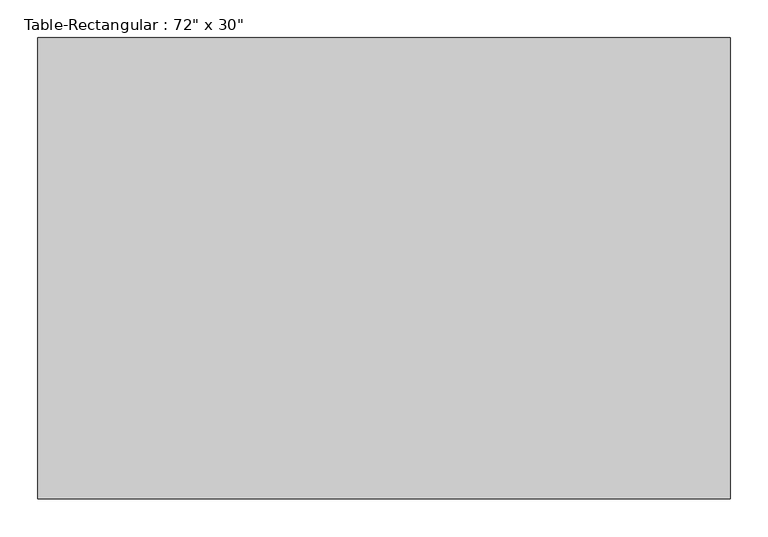
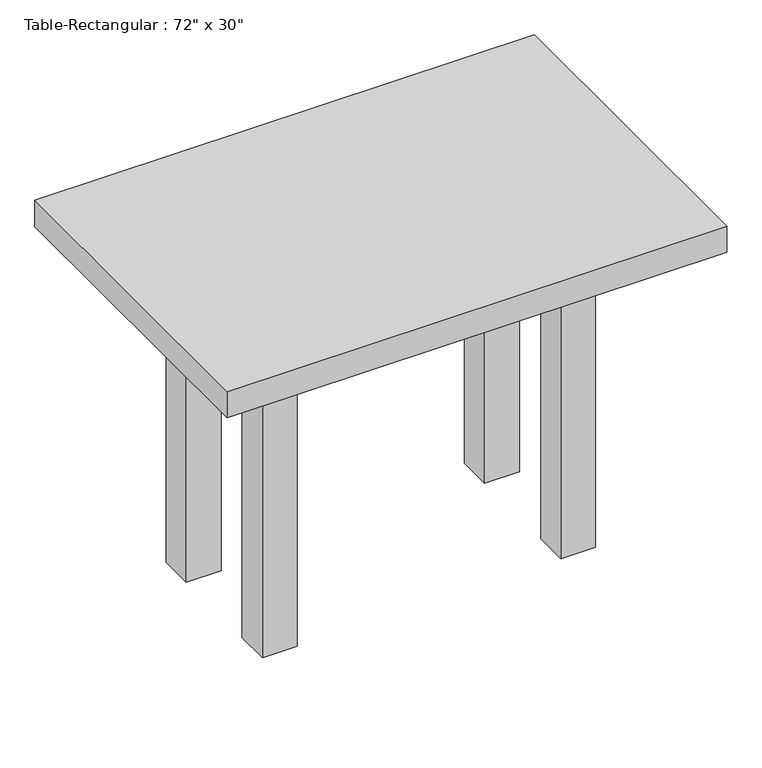
"""IFC4 building model written with IfcOpenShell, lengths in millimetres: furniture geometry."""

from ifc_helpers import new_model, si_unit, frame, origin, origin_with_axes, place, context, project, spatial, polyline, outline, extrude, source, transform, mapped, element, save


def furniture_5341d497(model_context):
    return source(origin(), model_context, "Body", "SweptSolid", [
        extrude(outline(polyline([(241.3, 114.3), (241.3, 88.9), (-241.3, 88.9), (-241.3, 114.3), (241.3, 114.3)])), frame((0.0, 0.0, 508.0), z_axis=(0.0, 0.0, 1.0), x_axis=(1.0, 0.0, 0.0)), (0.0, 0.0, 1.0), 101.6),
        extrude(outline(polyline([(241.3, -114.3), (-241.3, -114.3), (-241.3, -88.9), (241.3, -88.9), (241.3, -114.3)])), frame((0.0, 0.0, 508.0), z_axis=(0.0, 0.0, 1.0), x_axis=(1.0, 0.0, 0.0)), (0.0, 0.0, 1.0), 101.6),
        extrude(outline(polyline([(-254.0, -88.9), (-279.4, -88.9), (-279.4, 88.9), (-254.0, 88.9), (-254.0, -88.9)])), frame((0.0, 0.0, 508.0), z_axis=(0.0, 0.0, 1.0), x_axis=(1.0, 0.0, 0.0)), (0.0, 0.0, 1.0), 101.6),
        extrude(outline(polyline([(254.0, -88.9), (254.0, 88.9), (279.4, 88.9), (279.4, -88.9), (254.0, -88.9)])), frame((0.0, 0.0, 508.0), z_axis=(0.0, 0.0, 1.0), x_axis=(1.0, 0.0, 0.0)), (0.0, 0.0, 1.0), 101.6),
        extrude(outline(polyline([(457.2, 304.8), (457.2, -304.8), (-457.2, -304.8), (-457.2, 304.8), (457.2, 304.8)])), frame((0.0, 0.0, 609.6), z_axis=(0.0, 0.0, 1.0), x_axis=(1.0, 0.0, 0.0)), (0.0, 0.0, 1.0), 50.8),
        extrude(outline(polyline([(-241.3, 152.4), (-241.3, 88.9), (-304.8, 88.9), (-304.8, 152.4), (-241.3, 152.4)])), origin_with_axes(), (0.0, 0.0, 1.0), 609.6),
        extrude(outline(polyline([(241.3, 152.4), (304.8, 152.4), (304.8, 88.9), (241.3, 88.9), (241.3, 152.4)])), origin_with_axes(), (0.0, 0.0, 1.0), 609.6),
        extrude(outline(polyline([(-241.3, -152.4), (-304.8, -152.4), (-304.8, -88.9), (-241.3, -88.9), (-241.3, -152.4)])), origin_with_axes(), (0.0, 0.0, 1.0), 609.6),
        extrude(outline(polyline([(241.3, -152.4), (241.3, -88.9), (304.8, -88.9), (304.8, -152.4), (241.3, -152.4)])), origin_with_axes(), (0.0, 0.0, 1.0), 609.6),
    ])


if __name__ == "__main__":
    model = new_model("IFC4")
    model_context = context("Model", 3, world=origin())
    ifc_project = project(units=[si_unit("LENGTHUNIT", "METRE", prefix="MILLI")], contexts=[model_context])
    site = spatial("IfcSite", under=ifc_project)
    building = spatial("IfcBuilding", under=site)
    placement = place(None, origin())
    furniture_shape = furniture_5341d497(model_context)
    element("IfcFurniture", 1, ObjectType="Table-Rectangular : 72\" x 30\"", at=placement, inside=building, context=model_context, shape_type="MappedRepresentation", body=[
        mapped(furniture_shape, transform((0.0, 0.0, 0.0), x_axis=(1.0, 0.0, 0.0), y_axis=(0.0, 1.0, 0.0), z_axis=(0.0, 0.0, 1.0))),
    ])
    save(model, "model.ifc")

# Revit data of these elements
# Type "Table-Rectangular : 72\" x 30\""
#   Assembly Code = "E2020200"
#   Height = 2' - 2"
#   Length = 3' - 0"
#   Width = 2' - 0"
#   Base Material = Birch
#   Top Material = Birch
#   Default Elevation = 0
# Element 1 (IfcFurniture, "Table-Rectangular : 72\" x 30\"")
#   Materials on its faces: "Birch"
# Materials
#   "Birch": class "Wood", colour RGB 224 178 126, transparency 0, Description = "Betula Alleghaniensis", Cost = 0
